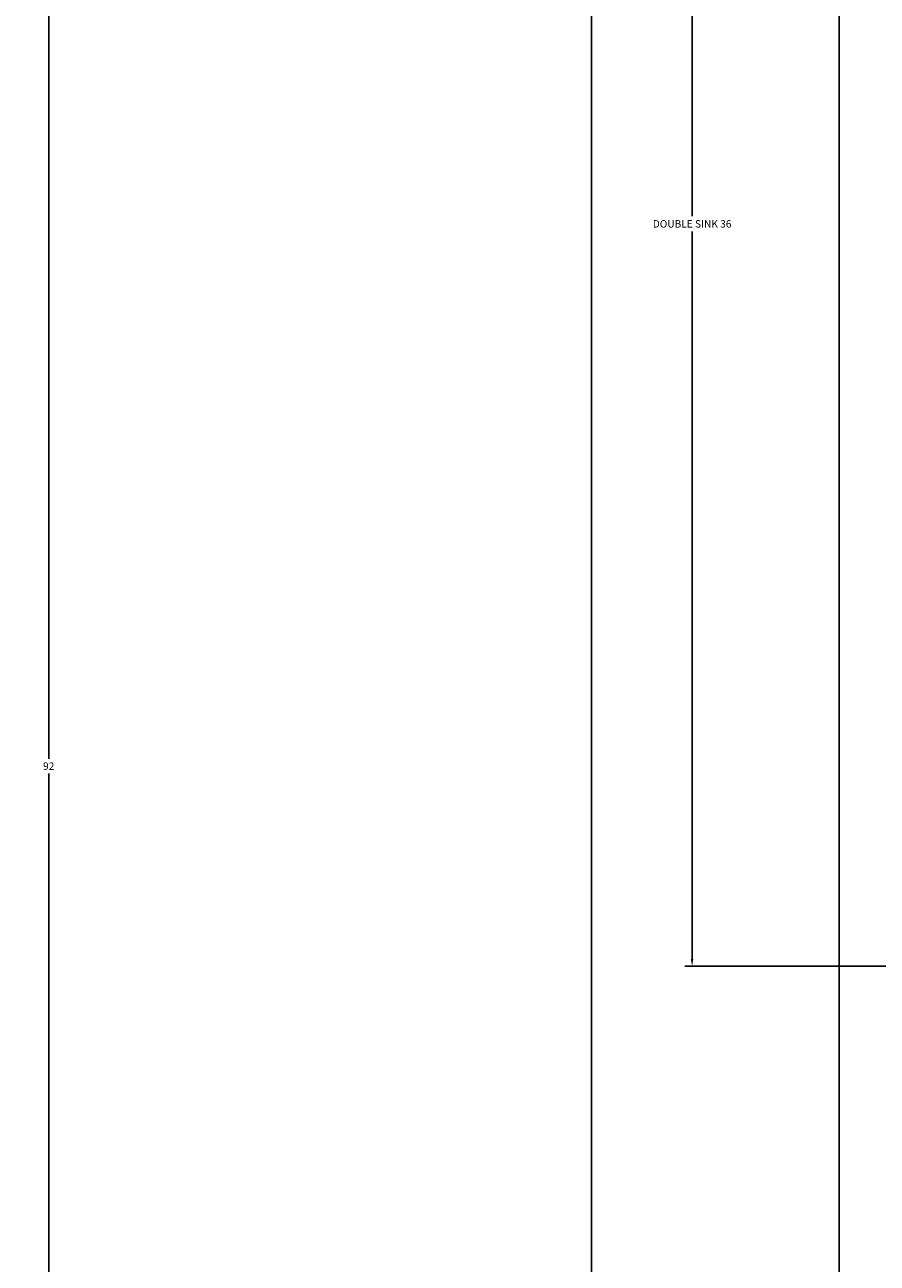
# Model space of a CAD drawing. Units: inches. Extents: x 2307 to 2544, y 2171 to 2540.
# Tile 35 of 52: x 2472 to 2493, y 2377 to 2407. Entities that reach past the tile are written whole.
import ezdxf

# ---------------------------------------------------------------- set-up
doc = ezdxf.new("R2010")
doc.units = ezdxf.units.IN
doc.layers.add('A-ANNO-DIMS', color=2, linetype='Continuous', lineweight=18)
doc.layers.add('A-FLOR-CASE', color=9, linetype='Continuous', lineweight=18)
doc.styles.get("Standard").update_dxf_attribs({"font": 'arial.ttf'})
doc.dimstyles.get("Standard").update_dxf_attribs({"dimtxt": 0.18, "dimasz": 0.18, "dimexe": 0.18, "dimexo": 0.0625, "dimgap": 0.09, "dimtad": 0, "dimtih": 1, "dimtoh": 1, "dimdec": 4, "dimzin": 0, "dimdsep": 46, "dimtxsty": 'Standard', "dimcen": 0.09, "dimadec": 0, "dimazin": 0, "dimtfac": 1, "dimtdec": 4, "dimtofl": 0, "dimtmove": 0, "dimatfit": 3, "dimfxl": 1, "dimtolj": 1, "dimtzin": 0, "dimarcsym": 0})

# ---------------------------------------------------------------- blocks, each defined once
blk = doc.blocks.new('*D32')
at = {"layer": 'A-ANNO-DIMS', "color": 0, "lineweight": -2, "transparency": 16777216}
for p, q in [((2493.473, 2420.657), (2487.956, 2420.657)), ((2488.136, 2420.477), (2488.136, 2402.84)), ((2488.136, 2384.837), (2488.136, 2402.474)), ((2493.473, 2384.657), (2487.956, 2384.657))]:
    blk.add_line(p, q, dxfattribs=at)
at = {"layer": 'A-ANNO-DIMS', "color": 0, "transparency": 16777216}
for points in [[(2488.106, 2420.477), (2488.166, 2420.477), (2488.136, 2420.657)], [(2488.106, 2384.837), (2488.166, 2384.837), (2488.136, 2384.657)]]:
    blk.add_solid(points, dxfattribs=at)
at = {"layer": 'Defpoints', "color": 0, "transparency": 16777216}
for p in [(2493.536, 2420.657), (2488.136, 2384.657), (2493.536, 2384.657)]:
    blk.add_point(p, dxfattribs=at)
at = {"layer": 'A-ANNO-DIMS', "color": 0, "transparency": 16777216, "insert": (2488.136, 2402.657), "char_height": 0.18, "attachment_point": 5}
blk.add_mtext('\\A1;DOUBLE SINK 36', dxfattribs=at)
blk = doc.blocks.new('*D49')
at = {"layer": 'A-ANNO-DIMS', "color": 0, "lineweight": -2, "transparency": 16777216}
for p, q in [((2491.633, 2435.51), (2472.366, 2435.51)), ((2472.546, 2435.33), (2472.546, 2389.691)), ((2472.546, 2343.69), (2472.546, 2389.328)), ((2491.633, 2343.51), (2472.366, 2343.51))]:
    blk.add_line(p, q, dxfattribs=at)
at = {"layer": 'A-ANNO-DIMS', "color": 0, "transparency": 16777216}
for points in [[(2472.516, 2435.33), (2472.576, 2435.33), (2472.546, 2435.51)], [(2472.516, 2343.69), (2472.576, 2343.69), (2472.546, 2343.51)]]:
    blk.add_solid(points, dxfattribs=at)
at = {"layer": 'Defpoints', "color": 0, "transparency": 16777216}
for p in [(2472.546, 2435.51), (2491.696, 2435.51), (2491.696, 2343.51)]:
    blk.add_point(p, dxfattribs=at)
at = {"layer": 'A-ANNO-DIMS', "color": 0, "transparency": 16777216, "insert": (2472.546, 2389.51), "char_height": 0.18, "attachment_point": 5}
blk.add_mtext('\\A1;92', dxfattribs=at)
blk = doc.blocks.new('*D54')
at = {"layer": 'A-ANNO-DIMS', "color": 0, "lineweight": -2, "transparency": 16777216}
for p, q in [((2461.696, 2435.447), (2461.696, 2171.18)), ((2491.696, 2435.447), (2491.696, 2171.18)), ((2461.876, 2171.36), (2476.477, 2171.36)), ((2491.516, 2171.36), (2476.914, 2171.36))]:
    blk.add_line(p, q, dxfattribs=at)
at = {"layer": 'A-ANNO-DIMS', "color": 0, "transparency": 16777216}
for points in [[(2461.876, 2171.39), (2461.876, 2171.33), (2461.696, 2171.36)], [(2491.516, 2171.39), (2491.516, 2171.33), (2491.696, 2171.36)]]:
    blk.add_solid(points, dxfattribs=at)
at = {"layer": 'Defpoints', "color": 0, "transparency": 16777216}
for p in [(2461.696, 2435.51), (2491.696, 2435.51), (2491.696, 2171.36)]:
    blk.add_point(p, dxfattribs=at)
at = {"layer": 'A-ANNO-DIMS', "color": 0, "transparency": 16777216, "insert": (2476.696, 2171.36), "char_height": 0.18, "attachment_point": 5}
blk.add_mtext('\\A1;30', dxfattribs=at)
blk = doc.blocks.new('*D59')
at = {"layer": 'A-ANNO-DIMS', "color": 0, "lineweight": -2, "transparency": 16777216}
for p, q in [((2455.696, 2315.572), (2455.696, 2540.345)), ((2455.876, 2540.165), (2470.477, 2540.165)), ((2485.516, 2540.165), (2470.914, 2540.165)), ((2485.696, 2315.572), (2485.696, 2540.345))]:
    blk.add_line(p, q, dxfattribs=at)
at = {"layer": 'A-ANNO-DIMS', "color": 0, "transparency": 16777216}
for points in [[(2455.876, 2540.195), (2455.876, 2540.135), (2455.696, 2540.165)], [(2485.516, 2540.195), (2485.516, 2540.135), (2485.696, 2540.165)]]:
    blk.add_solid(points, dxfattribs=at)
at = {"layer": 'Defpoints', "color": 0, "transparency": 16777216}
for p in [(2455.696, 2540.165), (2455.696, 2315.51), (2485.696, 2315.51)]:
    blk.add_point(p, dxfattribs=at)
at = {"layer": 'A-ANNO-DIMS', "color": 0, "transparency": 16777216, "insert": (2470.696, 2540.165), "char_height": 0.18, "attachment_point": 5}
blk.add_mtext('\\A1;30', dxfattribs=at)

msp = doc.modelspace()

# ---------------------------------------------------------------- linework, layer by layer
at = {"layer": 'A-FLOR-CASE'}
msp.add_line((2491.6958, 2435.5096), (2491.6958, 2343.5096), dxfattribs=at)

# ---------------------------------------------------------------- dimensions: what is measured, and where the dimension line sits
at = {"layer": 'A-ANNO-DIMS'}
for base, p1, p2, picture, middle in [((2455.6958, 2540.1649), (2485.6958, 2315.5096), (2455.6958, 2315.5096), '*D59', (2470.6958, 2540.1649)), ((2491.6958, 2171.3596), (2461.6958, 2435.5096), (2491.6958, 2435.5096), '*D54', (2476.6958, 2171.3596))]:
    dim = msp.add_linear_dim(base=base, p1=p1, p2=p2, dimstyle='Standard', override={"dimdec": 0, "dimlfac": 1, "dimrnd": 0, "dimzin": 0, "dimdsep": 46, "dimlunit": 2}, dxfattribs=at)
    dim.commit()
    dim.dimension.update_dxf_attribs({"geometry": picture, "text_midpoint": middle})
dim = msp.add_linear_dim(base=(2472.5458, 2435.5096), p1=(2491.6958, 2343.5096), p2=(2491.6958, 2435.5096), angle=90, dimstyle='Standard', override={"dimdec": 0, "dimlfac": 1, "dimrnd": 0, "dimzin": 0, "dimdsep": 46, "dimlunit": 2}, dxfattribs=at)
dim.commit()
dim.dimension.update_dxf_attribs({"geometry": '*D49', "text_midpoint": (2472.5458, 2389.5096)})
dim = msp.add_linear_dim(base=(2488.1356, 2384.6573), p1=(2493.5356, 2420.6573), p2=(2493.5356, 2384.6573), angle=270, text='DOUBLE SINK <>', dimstyle='Standard', override={"dimdec": 0, "dimlfac": 1, "dimrnd": 0, "dimzin": 0, "dimdsep": 46, "dimlunit": 2}, dxfattribs=at)
dim.commit()
dim.dimension.update_dxf_attribs({"geometry": '*D32', "text_midpoint": (2488.1356, 2402.6573)})

doc.saveas('drawing.dxf')
